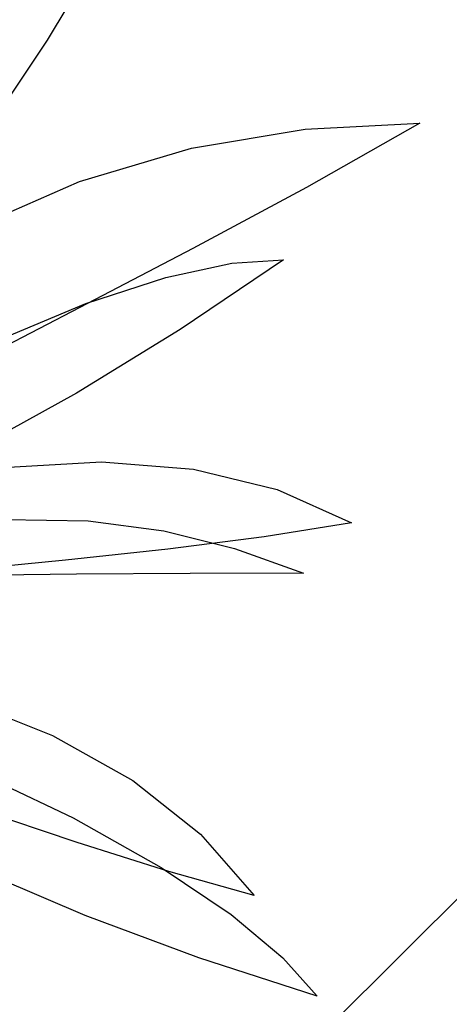
# Model space of a CAD drawing. Units: inches. Extents: x 3590 to 5167, y 65 to 1917.
# Tile 94 of 100: x 5058.39 to 5065.29, y 1773.22 to 1789.03. Entities that reach past the tile are written whole.
import ezdxf

# ---------------------------------------------------------------- set-up
doc = ezdxf.new("R2010")
doc.units = ezdxf.units.IN
for name, color, linetype, lineweight in [('A-ANNO-DIMS', 2, 'Continuous', 18), ('A-FLOR-PATT', 8, 'Continuous', 13), ('L-PLNT', 94, 'Continuous', 18)]:
    doc.layers.add(name, color=color, linetype=linetype, lineweight=lineweight)
doc.layers.add('DIENHOA', color=3, linetype='Continuous')
doc.styles.get("Standard").update_dxf_attribs({"font": 'arial.ttf'})
doc.dimstyles.new('ISO-25', dxfattribs={"dimtxt": 9, "dimasz": 2.5, "dimexe": 1.25, "dimexo": 0.625, "dimtad": 1, "dimdec": 1, "dimlunit": 3, "dimtxsty": 'Standard', "dimcen": 2.5, "dimadec": 0, "dimazin": 0, "dimtfac": 1, "dimtdec": 1, "dimtmove": 0, "dimatfit": 3, "dimfxl": 1, "dimarcsym": 0})

# ---------------------------------------------------------------- blocks, each defined once
blk = doc.blocks.new('Cay03_mb')
at = {"layer": 'DIENHOA'}
for p, q in [((436.81, 297.21), (510.97, 309.61)), ((510.97, 309.61), (585.91, 313.53)), ((585.91, 313.53), (511.78, 271.41)), ((363.38, 275.41), (436.81, 297.21)), ((290.63, 243.24), (363.38, 275.41)), ((511.78, 271.41), (437.63, 231.46)), ((437.63, 231.46), (363.69, 192.89)), ((363.69, 192.89), (290.19, 154.87)), ((314.63, 54.14), (369.18, 53.28)), ((369.18, 53.28), (418.6, 46.82)), ((418.6, 46.82), (464.87, 35.24)), ((464.87, 35.24), (510, 19)), ((361.61, 18.5), (289.03, 17.44)), ((435.8, 18.92), (361.61, 18.5)), ((510, 19), (435.8, 18.92)), ((289.55, -107.64), (359.29, -141.1)), ((359.29, -141.1), (416.89, -173.51)), ((416.89, -173.51), (462.55, -204.2)), ((367.1, -204.83), (296, -174.69)), ((441.55, -232.67), (367.1, -204.83)), ((462.55, -204.2), (496.5, -232.48)), ((518.93, -257.68), (441.55, -232.67)), ((496.5, -232.48), (518.93, -257.68))]:
    blk.add_line(p, q, dxfattribs=at)
for points in [[(384.28, 437.45), (342.25, 367.83), (298.14, 301.71), (252.56, 239.37), (206.11, 181.11), (159.39, 127.21), (113.01, 77.96), (67.57, 33.64), (23.69, -5.44)], [(496.74, 224.01), (429.38, 178.44), (361.6, 136.93), (294.07, 99.46), (227.46, 66.07), (162.44, 36.74), (99.68, 11.49), (39.84, -9.67), (-16.39, -26.73)], [(-16.39, -26.73), (75.38, 37.88), (160.06, 91.82), (237.27, 135.67), (306.57, 170.01), (367.58, 195.44), (419.88, 212.52), (463.07, 221.85), (496.74, 224.01)], [(23.69, -5.44), (99.27, 29.67), (173.22, 57.09), (244.79, 76.69), (313.26, 88.31), (377.88, 91.81), (437.93, 87.02), (492.67, 73.8), (541.37, 52)], [(541.37, 52), (484.11, 42.89), (421.18, 34.83), (354.36, 27.58), (285.41, 20.89), (216.1, 14.49), (148.2, 8.14), (83.47, 1.58), (23.69, -5.44)], [(-16.39, -26.73), (66.95, -26.58), (145.58, -32.71), (218.77, -44.94), (285.79, -63.12), (345.92, -87.06), (398.42, -116.6), (442.57, -151.57), (477.63, -191.79)], [(477.63, -191.79), (421.82, -176.03), (361.32, -156.94), (297.62, -135.49), (232.22, -112.64), (166.63, -89.37), (102.33, -66.65), (40.82, -45.45), (-16.39, -26.73)]]:
    blk.add_lwpolyline(points, dxfattribs=at)
blk = doc.blocks.new('*D322')
at = {"layer": 'A-ANNO-DIMS', "color": 0, "lineweight": -2, "transparency": 16777216}
for p, q in [((5035.744, 1766.184), (5035.744, 1761.199)), ((5064.812, 1766.184), (5064.812, 1761.199)), ((5038.244, 1762.449), (5062.312, 1762.449)), ((5064.812, 1762.449), (5166.991, 1762.449))]:
    blk.add_line(p, q, dxfattribs=at)
at = {"layer": 'A-ANNO-DIMS', "color": 0, "transparency": 16777216}
for points in [[(5038.244, 1762.866), (5038.244, 1762.032), (5035.744, 1762.449)], [(5062.312, 1762.866), (5062.312, 1762.032), (5064.812, 1762.449)]]:
    blk.add_solid(points, dxfattribs=at)
at = {"layer": 'Defpoints', "color": 0, "transparency": 16777216}
for p in [(5035.744, 1766.809), (5064.812, 1766.809), (5064.812, 1762.449)]:
    blk.add_point(p, dxfattribs=at)
at = {"layer": 'A-ANNO-DIMS', "color": 0, "transparency": 16777216, "insert": (5117.152, 1767.669), "char_height": 9, "attachment_point": 5}
blk.add_mtext('PLANT 2\'-5" TYP.', dxfattribs=at)
blk = doc.blocks.new('*D323')
at = {"layer": 'A-ANNO-DIMS', "color": 0, "lineweight": -2, "transparency": 16777216}
for p, q in [((5069.172, 1795.216), (5069.172, 1874.95)), ((5065.437, 1795.216), (5070.422, 1795.216)), ((5069.172, 1769.309), (5069.172, 1792.716)), ((5065.437, 1766.809), (5070.422, 1766.809))]:
    blk.add_line(p, q, dxfattribs=at)
at = {"layer": 'A-ANNO-DIMS', "color": 0, "transparency": 16777216}
for points in [[(5068.756, 1792.716), (5069.589, 1792.716), (5069.172, 1795.216)], [(5068.756, 1769.309), (5069.589, 1769.309), (5069.172, 1766.809)]]:
    blk.add_solid(points, dxfattribs=at)
at = {"layer": 'Defpoints', "color": 0, "transparency": 16777216}
for p in [(5064.812, 1795.216), (5069.172, 1795.216), (5064.812, 1766.809)]:
    blk.add_point(p, dxfattribs=at)
at = {"layer": 'A-ANNO-DIMS', "color": 0, "transparency": 16777216, "insert": (5063.894, 1836.333), "char_height": 9, "attachment_point": 5, "rotation": 90}
blk.add_mtext('2\'-4 1/2" TYP.', dxfattribs=at)

msp = doc.modelspace()

# ---------------------------------------------------------------- hatches: boundary and pattern name
at = {"layer": 'A-FLOR-PATT', "transparency": 33554687}
h = msp.add_hatch(dxfattribs=at)
h.set_pattern_fill('AR-HBONE', color=256, scale=0.2)
h.set_pattern_definition([(45, (-588.972, 0), (0, 28.73682), [60.96, -20.32]), (135, (-574.604, 14.368), (3e-15, 28.73682), [60.96, -20.32])])
h.paths.add_polyline_path([(5071.274, 1796.999), (4933.274, 1796.999), (4933.274, 1753.999), (4962.774, 1753.999, -0.414214), (4928.774, 1719.999), (4933.274, 1718.999), (4933.274, 1334.999), (5071.274, 1334.999)])
h.paths.add_polyline_path([(4951.78, 1521.077), (4951.715, 1521.04), (4951.563, 1520.895)], flags=16)
h.paths.add_polyline_path([(4952.267, 1521.376), (4952.198, 1521.371), (4952.198, 1521.356)], flags=0)
h.paths.add_polyline_path([(4967.051, 1529.728), (4965.231, 1528.694), (4963.411, 1527.714), (4961.756, 1526.851), (4963.589, 1527.449), (4964.036, 1527.478), (4962.975, 1527.249), (4961.76, 1526.852), (4959.792, 1525.834), (4958.005, 1524.895), (4956.24, 1523.93), (4954.504, 1522.919), (4954.129, 1522.682), (4953.361, 1521.997), (4953.366, 1521.998), (4953.605, 1522.064), (4955.106, 1522.761), (4956.921, 1523.434), (4958.678, 1523.915), (4960.358, 1524.2), (4961.945, 1524.286), (4964.171, 1524.108), (4965.958, 1523.309), (4963.863, 1522.976), (4965.187, 1522.499), (4963.366, 1522.497), (4961.545, 1522.487), (4959.764, 1522.461), (4958.304, 1522.419), (4957.974, 1522.388), (4956.307, 1522.232), (4954.718, 1522.071), (4953.251, 1521.899), (4953.525, 1521.623), (4954.331, 1521.379), (4956.243, 1521.23), (4958.039, 1520.93), (4959.684, 1520.483), (4961.16, 1519.896), (4963.107, 1518.8), (4964.393, 1517.325), (4962.973, 1517.726), (4964.558, 1516.661), (4965.407, 1515.708), (4963.507, 1516.322), (4961.68, 1517.005), (4959.935, 1517.745), (4958.282, 1518.528), (4956.732, 1519.343), (4955.295, 1520.175), (4954.672, 1520.572), (4954.513, 1520.627), (4955.658, 1519.318), (4956.703, 1517.982), (4957.644, 1516.647), (4958.485, 1515.334), (4959.55, 1513.524), (4960.438, 1511.769), (4958.841, 1513.62), (4957.452, 1515.325), (4955.819, 1517.459), (4956.665, 1515.448), (4957.111, 1513.923), (4957.447, 1511.714), (4957.076, 1509.793), (4956.538, 1511.11), (4955.992, 1512.569), (4955.444, 1514.125), (4954.898, 1515.735), (4954.357, 1517.356), (4953.824, 1518.943), (4953.305, 1520.452), (4953.065, 1521.116), (4952.971, 1521.146), (4952.949, 1521.086), (4952.73, 1520.199), (4953.37, 1518.024), (4953.757, 1516.373), (4954.051, 1514.765), (4954.264, 1513.221), (4954.471, 1511.131), (4954.497, 1510.402), (4954.409, 1511.76), (4954.264, 1513.221), (4954.051, 1514.765), (4953.757, 1516.373), (4953.37, 1518.024), (4952.877, 1519.698), (4952.716, 1520.141), (4952.533, 1519.059), (4952.374, 1517.789), (4952.219, 1516.312), (4952.046, 1514.6), (4951.833, 1512.626), (4951.557, 1510.363), (4951.203, 1512.168), (4950.852, 1514.339), (4950.985, 1516.376), (4951.66, 1518.286), (4952.593, 1520.481), (4952.357, 1521.13), (4951.855, 1520.328), (4950.839, 1518.908), (4949.777, 1517.587), (4948.916, 1516.617), (4948.111, 1515.256), (4947.089, 1513.554), (4945.889, 1511.615), (4946.326, 1513.402), (4946.562, 1514.249), (4945.528, 1513.327), (4944.581, 1512.531), (4946.018, 1514.508), (4947.204, 1516.048), (4947.893, 1517.313), (4949.307, 1518.764), (4950.414, 1519.767), (4950.451, 1519.806), (4952.267, 1521.376), (4951.645, 1521.493), (4950.404, 1521.18), (4948.044, 1520.359), (4946.119, 1519.452), (4944.572, 1518.475), (4943.35, 1517.443), (4941.997, 1515.92), (4941.661, 1515.275), (4942.813, 1516.99), (4944.572, 1518.475), (4946.119, 1519.452), (4948.044, 1520.359), (4950.404, 1521.18), (4951.645, 1521.493), (4949.647, 1521.868), (4948.6, 1521.756), (4947.126, 1521.57), (4945.42, 1521.348), (4943.45, 1521.105), (4941.183, 1520.856), (4942.86, 1521.613), (4943.873, 1522.03), (4942.952, 1521.909), (4941.41, 1521.485), (4939.543, 1520.67), (4938.968, 1520.226), (4940.733, 1521.299), (4942.952, 1521.909), (4943.702, 1522.008), (4945.894, 1522.7), (4947.565, 1522.714), (4948.921, 1522.566), (4951.131, 1522.183), (4950.971, 1522.297), (4948.129, 1523.006), (4946.035, 1523.707), (4944.232, 1524.521), (4942.707, 1525.461), (4941.444, 1526.537), (4940.43, 1527.761), (4939.649, 1529.143), (4941.421, 1528.122), (4943.147, 1527.132), (4944.841, 1526.175), (4946.514, 1525.25), (4948.179, 1524.359), (4948.365, 1524.263), (4946.475, 1526.045), (4945.181, 1527.54), (4944.19, 1529.033), (4943.496, 1530.54), (4943.278, 1531.36), (4942.498, 1531.919), (4943.114, 1531.762), (4942.959, 1533.659), (4944.14, 1531.989), (4944.612, 1531.323), (4946.202, 1530.463), (4947.486, 1529.509), (4948.79, 1528.226), (4950.368, 1526.237), (4949.485, 1528.155), (4948.851, 1530.123), (4948.491, 1532.041), (4948.381, 1533.918), (4948.501, 1535.76), (4948.827, 1537.573), (4949.418, 1535.565), (4949.957, 1533.569), (4950.464, 1531.586), (4950.961, 1529.617), (4951.391, 1527.954), (4951.724, 1530.687), (4952.201, 1532.58), (4952.889, 1534.33), (4953.77, 1535.951), (4954.827, 1537.46), (4954.521, 1535.39), (4954.273, 1533.937), (4955.58, 1535.663), (4956.748, 1536.739), (4956.159, 1534.78), (4955.589, 1532.873), (4955.043, 1531.006), (4954.525, 1529.166), (4954.038, 1527.341), (4953.638, 1525.733), (4953.611, 1525.586), (4953.398, 1524.166), (4953.382, 1524.009), (4954.07, 1525.476), (4954.912, 1527.022), (4956.136, 1528.894), (4957.847, 1530.577), (4959.376, 1531.54), (4958.256, 1530.104), (4957.143, 1528.663), (4956.066, 1527.243), (4955.056, 1525.871), (4954.141, 1524.571), (4953.352, 1523.372), (4953.311, 1523.303), (4953.273, 1522.925), (4953.261, 1522.382), (4954.103, 1523.373), (4954.63, 1524.284), (4955.961, 1526.358), (4957.23, 1528.13), (4958.421, 1529.609), (4960.037, 1531.368), (4961.374, 1532.375), (4962.101, 1532.77), (4961.07, 1531.061), (4959.987, 1529.438), (4958.869, 1527.908), (4958.15, 1527.007), (4959.803, 1528.003), (4961.589, 1528.793), (4963.391, 1529.328), (4965.211, 1529.632)], flags=16)
h.paths.add_polyline_path([(4962.944, 1523.182), (4961.107, 1523.422), (4960.392, 1523.362), (4962.35, 1523.331)], flags=0)
h.paths.add_polyline_path([(5049.541, 1584.551), (5049.476, 1584.515), (5049.325, 1584.37)], flags=16)
h.paths.add_polyline_path([(5050.028, 1584.851), (5049.959, 1584.845), (5049.959, 1584.83)], flags=0)
h.paths.add_polyline_path([(5042.333, 1581.949), (5043.88, 1582.926), (5045.806, 1583.833), (5048.165, 1584.654), (5049.406, 1584.967), (5047.408, 1585.342), (5046.361, 1585.231), (5044.888, 1585.044), (5043.181, 1584.822), (5041.211, 1584.579), (5038.944, 1584.33), (5040.622, 1585.087), (5041.634, 1585.504), (5040.713, 1585.383), (5039.171, 1584.959), (5037.304, 1584.144), (5036.729, 1583.7), (5038.494, 1584.773), (5040.713, 1585.383), (5041.463, 1585.482), (5043.655, 1586.174), (5045.326, 1586.188), (5046.682, 1586.04), (5048.893, 1585.657), (5048.732, 1585.771), (5045.891, 1586.48), (5043.796, 1587.181), (5041.994, 1587.996), (5040.468, 1588.935), (5039.205, 1590.011), (5038.191, 1591.235), (5037.41, 1592.617), (5039.182, 1591.596), (5040.909, 1590.607), (5042.602, 1589.649), (5044.275, 1588.724), (5045.94, 1587.833), (5046.126, 1587.738), (5044.237, 1589.519), (5042.942, 1591.015), (5041.952, 1592.508), (5041.257, 1594.014), (5041.039, 1594.834), (5040.26, 1595.393), (5040.875, 1595.237), (5040.721, 1597.133), (5041.901, 1595.463), (5042.373, 1594.798), (5043.963, 1593.938), (5045.247, 1592.983), (5046.552, 1591.701), (5048.129, 1589.712), (5047.247, 1591.63), (5046.613, 1593.597), (5046.252, 1595.515), (5046.142, 1597.392), (5046.262, 1599.234), (5046.588, 1601.047), (5047.179, 1599.039), (5047.718, 1597.043), (5048.225, 1595.06), (5048.722, 1593.091), (5049.152, 1591.429), (5049.485, 1594.161), (5049.962, 1596.054), (5050.65, 1597.804), (5051.532, 1599.425), (5052.589, 1600.934), (5052.283, 1598.864), (5052.034, 1597.411), (5053.341, 1599.137), (5054.509, 1600.213), (5053.92, 1598.254), (5053.35, 1596.348), (5052.805, 1594.48), (5052.286, 1592.64), (5051.799, 1590.815), (5051.4, 1589.207), (5051.373, 1589.06), (5051.159, 1587.64), (5051.143, 1587.483), (5051.831, 1588.95), (5052.673, 1590.496), (5053.898, 1592.368), (5055.608, 1594.051), (5057.137, 1595.014), (5056.017, 1593.578), (5054.904, 1592.137), (5053.828, 1590.717), (5052.817, 1589.345), (5051.902, 1588.046), (5051.113, 1586.846), (5051.072, 1586.777), (5051.034, 1586.399), (5051.022, 1585.856), (5051.864, 1586.847), (5052.391, 1587.758), (5053.723, 1589.832), (5054.991, 1591.604), (5056.182, 1593.083), (5057.798, 1594.842), (5059.135, 1595.849), (5059.863, 1596.244), (5058.831, 1594.535), (5057.749, 1592.912), (5056.63, 1591.382), (5055.912, 1590.482), (5057.564, 1591.477), (5059.35, 1592.267), (5061.152, 1592.802), (5062.972, 1593.106), (5064.812, 1593.203), (5062.992, 1592.169), (5061.172, 1591.188), (5059.518, 1590.325), (5061.35, 1590.924), (5061.797, 1590.952), (5060.737, 1590.723), (5059.521, 1590.326), (5057.553, 1589.308), (5055.766, 1588.369), (5054.002, 1587.404), (5052.265, 1586.393), (5051.891, 1586.156), (5051.122, 1585.471), (5051.127, 1585.472), (5051.366, 1585.538), (5052.867, 1586.235), (5054.682, 1586.908), (5056.439, 1587.389), (5058.12, 1587.675), (5059.706, 1587.76), (5061.933, 1587.583), (5063.719, 1586.783), (5061.624, 1586.45), (5062.949, 1585.973), (5061.127, 1585.971), (5059.307, 1585.961), (5057.525, 1585.935), (5056.065, 1585.893), (5055.735, 1585.862), (5054.068, 1585.707), (5052.479, 1585.546), (5051.012, 1585.373), (5051.286, 1585.097), (5052.092, 1584.853), (5054.004, 1584.704), (5055.8, 1584.404), (5057.446, 1583.958), (5058.921, 1583.37), (5060.868, 1582.274), (5062.154, 1580.799), (5060.734, 1581.2), (5062.32, 1580.135), (5063.168, 1579.182), (5061.269, 1579.796), (5059.441, 1580.479), (5057.696, 1581.219), (5056.043, 1582.003), (5054.493, 1582.817), (5053.057, 1583.649), (5052.433, 1584.047), (5052.274, 1584.101), (5053.42, 1582.793), (5054.464, 1581.457), (5055.405, 1580.121), (5056.247, 1578.809), (5057.311, 1576.998), (5058.199, 1575.244), (5056.602, 1577.094), (5055.213, 1578.799), (5053.58, 1580.933), (5054.427, 1578.922), (5054.872, 1577.397), (5055.208, 1575.189), (5054.838, 1573.267), (5054.299, 1574.584), (5053.754, 1576.043), (5053.206, 1577.599), (5052.659, 1579.209), (5052.118, 1580.83), (5051.585, 1582.417), (5051.066, 1583.927), (5050.826, 1584.59), (5050.733, 1584.62), (5050.711, 1584.561), (5050.491, 1583.673), (5051.131, 1581.498), (5051.518, 1579.847), (5051.813, 1578.24), (5052.026, 1576.695), (5052.233, 1574.605), (5052.258, 1573.876), (5052.17, 1575.234), (5052.026, 1576.695), (5051.813, 1578.24), (5051.518, 1579.847), (5051.131, 1581.498), (5050.638, 1583.172), (5050.477, 1583.615), (5050.294, 1582.533), (5050.136, 1581.263), (5049.981, 1579.786), (5049.807, 1578.074), (5049.594, 1576.1), (5049.318, 1573.837), (5048.965, 1575.642), (5048.613, 1577.813), (5048.747, 1579.85), (5049.421, 1581.76), (5050.354, 1583.955), (5050.118, 1584.604), (5049.616, 1583.802), (5048.6, 1582.382), (5047.538, 1581.061), (5046.677, 1580.091), (5045.872, 1578.73), (5044.85, 1577.028), (5043.651, 1575.089), (5044.087, 1576.877), (5044.324, 1577.723), (5043.289, 1576.801), (5042.342, 1576.005), (5043.779, 1577.982), (5044.966, 1579.522), (5045.655, 1580.787), (5047.068, 1582.239), (5048.175, 1583.241), (5048.213, 1583.28), (5050.028, 1584.851), (5049.406, 1584.967), (5048.165, 1584.654), (5045.806, 1583.833), (5043.88, 1582.926), (5042.333, 1581.949), (5041.111, 1580.917), (5039.758, 1579.394), (5039.423, 1578.749), (5040.575, 1580.464)], flags=16)
h.paths.add_polyline_path([(4954.799, 1533.12), (4954.262, 1532.079), (4953.831, 1530.935), (4953.505, 1529.636), (4953.283, 1528.133), (4953.167, 1526.376), (4953.156, 1524.315), (4953.277, 1521.236), (4952.802, 1521.842), (4951.557, 1521.998), (4950.976, 1521.961), (4952.661, 1521.941), (4952.802, 1521.842), (4953.152, 1523.593), (4953.167, 1526.376), (4953.283, 1528.133), (4953.609, 1530.346), (4954.456, 1532.592)], flags=0)
h.paths.add_polyline_path([(5050.563, 1585.316), (5049.318, 1585.472), (5048.737, 1585.435), (5050.422, 1585.415), (5050.563, 1585.316), (5050.914, 1587.067), (5050.928, 1589.851), (5051.045, 1591.607), (5051.371, 1593.82), (5052.217, 1596.066), (5052.56, 1596.594), (5052.024, 1595.554), (5051.592, 1594.409), (5051.266, 1593.11), (5051.045, 1591.607), (5050.928, 1589.851), (5050.918, 1587.789), (5051.038, 1584.71)], flags=0)
h.paths.add_polyline_path([(5058.153, 1586.836), (5060.111, 1586.805), (5060.705, 1586.656), (5058.868, 1586.896)], flags=0)
h.paths.add_polyline_path([(5049.541, 1430.936), (5049.476, 1430.9), (5049.325, 1430.755)], flags=16)
h.paths.add_polyline_path([(5050.028, 1431.236), (5049.959, 1431.231), (5049.959, 1431.215)], flags=0)
h.paths.add_polyline_path([(5046.588, 1447.432), (5047.179, 1445.425), (5047.718, 1443.429), (5048.225, 1441.446), (5048.722, 1439.476), (5049.152, 1437.814), (5049.485, 1440.546), (5049.962, 1442.439), (5050.65, 1444.189), (5051.532, 1445.811), (5052.589, 1447.319), (5052.283, 1445.249), (5052.034, 1443.796), (5053.341, 1445.522), (5054.509, 1446.598), (5053.92, 1444.64), (5053.35, 1442.733), (5052.805, 1440.865), (5052.286, 1439.025), (5051.799, 1437.201), (5051.4, 1435.592), (5051.373, 1435.445), (5051.159, 1434.025), (5051.143, 1433.868), (5051.831, 1435.335), (5052.673, 1436.881), (5053.898, 1438.753), (5055.608, 1440.436), (5057.137, 1441.4), (5056.017, 1439.963), (5054.904, 1438.522), (5053.828, 1437.102), (5052.817, 1435.73), (5051.902, 1434.431), (5051.113, 1433.231), (5051.072, 1433.162), (5051.034, 1432.784), (5051.022, 1432.242), (5051.864, 1433.232), (5052.391, 1434.143), (5053.723, 1436.217), (5054.991, 1437.989), (5056.182, 1439.468), (5057.798, 1441.227), (5059.135, 1442.235), (5059.863, 1442.629), (5058.831, 1440.921), (5057.749, 1439.298), (5056.63, 1437.767), (5055.912, 1436.867), (5057.564, 1437.863), (5059.35, 1438.652), (5061.152, 1439.187), (5062.972, 1439.491), (5064.812, 1439.588), (5062.992, 1438.554), (5061.172, 1437.573), (5059.518, 1436.71), (5061.35, 1437.309), (5061.797, 1437.337), (5060.737, 1437.108), (5059.521, 1436.711), (5057.553, 1435.693), (5055.766, 1434.754), (5054.002, 1433.789), (5052.265, 1432.778), (5051.891, 1432.541), (5051.122, 1431.856), (5051.127, 1431.857), (5051.366, 1431.923), (5052.867, 1432.62), (5054.682, 1433.293), (5056.439, 1433.775), (5058.12, 1434.06), (5059.706, 1434.145), (5061.933, 1433.968), (5063.719, 1433.168), (5061.624, 1432.835), (5062.949, 1432.358), (5061.127, 1432.357), (5059.307, 1432.346), (5057.525, 1432.32), (5056.065, 1432.278), (5055.735, 1432.248), (5054.068, 1432.092), (5052.479, 1431.931), (5051.012, 1431.759), (5051.286, 1431.482), (5052.092, 1431.238), (5054.004, 1431.089), (5055.8, 1430.789), (5057.446, 1430.343), (5058.921, 1429.755), (5060.868, 1428.66), (5062.154, 1427.185), (5060.734, 1427.585), (5062.32, 1426.52), (5063.168, 1425.567), (5061.269, 1426.181), (5059.441, 1426.865), (5057.696, 1427.604), (5056.043, 1428.388), (5054.493, 1429.202), (5053.057, 1430.034), (5052.433, 1430.432), (5052.274, 1430.487), (5053.42, 1429.178), (5054.464, 1427.842), (5055.405, 1426.506), (5056.247, 1425.194), (5057.311, 1423.383), (5058.199, 1421.629), (5056.602, 1423.479), (5055.213, 1425.184), (5053.58, 1427.318), (5054.427, 1425.307), (5054.872, 1423.782), (5055.208, 1421.574), (5054.838, 1419.652), (5054.299, 1420.97), (5053.754, 1422.428), (5053.206, 1423.984), (5052.659, 1425.595), (5052.118, 1427.215), (5051.585, 1428.802), (5051.066, 1430.312), (5050.826, 1430.975), (5050.733, 1431.005), (5050.711, 1430.946), (5050.491, 1430.058), (5051.131, 1427.883), (5051.518, 1426.232), (5051.813, 1424.625), (5052.026, 1423.081), (5052.233, 1420.991), (5052.258, 1420.261), (5052.17, 1421.619), (5052.026, 1423.081), (5051.813, 1424.625), (5051.518, 1426.232), (5051.131, 1427.883), (5050.638, 1429.558), (5050.477, 1430.001), (5050.294, 1428.918), (5050.136, 1427.648), (5049.981, 1426.171), (5049.807, 1424.459), (5049.594, 1422.485), (5049.318, 1420.222), (5048.965, 1422.028), (5048.613, 1424.199), (5048.747, 1426.235), (5049.421, 1428.146), (5050.354, 1430.34), (5050.118, 1430.989), (5049.616, 1430.187), (5048.6, 1428.768), (5047.538, 1427.446), (5046.677, 1426.477), (5045.872, 1425.116), (5044.85, 1423.413), (5043.651, 1421.474), (5044.087, 1423.262), (5044.324, 1424.109), (5043.289, 1423.186), (5042.342, 1422.391), (5043.779, 1424.368), (5044.966, 1425.907), (5045.655, 1427.173), (5047.068, 1428.624), (5048.175, 1429.627), (5048.213, 1429.666), (5050.028, 1431.236), (5049.406, 1431.353), (5048.165, 1431.039), (5045.806, 1430.218), (5043.88, 1429.311), (5042.333, 1428.334), (5041.111, 1427.302), (5039.758, 1425.779), (5039.423, 1425.134), (5040.575, 1426.849), (5042.333, 1428.334), (5043.88, 1429.311), (5045.806, 1430.218), (5048.165, 1431.039), (5049.406, 1431.353), (5047.408, 1431.727), (5046.361, 1431.616), (5044.888, 1431.429), (5043.181, 1431.207), (5041.211, 1430.964), (5038.944, 1430.715), (5040.622, 1431.472), (5041.634, 1431.89), (5040.713, 1431.769), (5039.171, 1431.345), (5037.304, 1430.53), (5036.729, 1430.085), (5038.494, 1431.158), (5040.713, 1431.769), (5041.463, 1431.867), (5043.655, 1432.559), (5045.326, 1432.573), (5046.682, 1432.425), (5048.893, 1432.042), (5048.732, 1432.156), (5045.891, 1432.865), (5043.796, 1433.566), (5041.994, 1434.381), (5040.468, 1435.321), (5039.205, 1436.396), (5038.191, 1437.62), (5037.41, 1439.002), (5039.182, 1437.982), (5040.909, 1436.992), (5042.602, 1436.034), (5044.275, 1435.109), (5045.94, 1434.218), (5046.126, 1434.123), (5044.237, 1435.904), (5042.942, 1437.4), (5041.952, 1438.893), (5041.257, 1440.399), (5041.039, 1441.219), (5040.26, 1441.778), (5040.875, 1441.622), (5040.721, 1443.518), (5041.901, 1441.848), (5042.373, 1441.183), (5043.963, 1440.323), (5045.247, 1439.369), (5046.552, 1438.086), (5048.129, 1436.097), (5047.247, 1438.015), (5046.613, 1439.982), (5046.252, 1441.901), (5046.142, 1443.778), (5046.262, 1445.619)], flags=16)
h.paths.add_polyline_path([(5052.382, 1444.255), (5051.623, 1442.78), (5052.024, 1441.939), (5052.56, 1442.98)], flags=0)
h.paths.add_polyline_path([(5050.563, 1431.701), (5049.318, 1431.857), (5048.737, 1431.821), (5050.422, 1431.8)], flags=0)
h.paths.add_polyline_path([(5058.153, 1433.221), (5060.111, 1433.19), (5060.705, 1433.041), (5058.868, 1433.281)], flags=0)
h.paths.add_polyline_path([(5049.541, 1352.285), (5049.476, 1352.249), (5049.325, 1352.104)], flags=16)
h.paths.add_polyline_path([(5050.028, 1352.585), (5049.959, 1352.58), (5049.959, 1352.564)], flags=0)
h.paths.add_polyline_path([(5046.588, 1368.781), (5047.179, 1366.774), (5047.718, 1364.778), (5048.225, 1362.795), (5048.722, 1360.825), (5049.152, 1359.163), (5049.485, 1361.896), (5049.962, 1363.789), (5050.65, 1365.538), (5051.532, 1367.16), (5052.589, 1368.669), (5052.283, 1366.598), (5052.034, 1365.145), (5053.341, 1366.871), (5054.509, 1367.947), (5053.92, 1365.989), (5053.35, 1364.082), (5052.805, 1362.214), (5052.286, 1360.374), (5051.799, 1358.55), (5051.4, 1356.942), (5051.373, 1356.794), (5051.159, 1355.374), (5051.143, 1355.218), (5051.831, 1356.684), (5052.673, 1358.23), (5053.898, 1360.102), (5055.608, 1361.786), (5057.137, 1362.749), (5056.017, 1361.313), (5054.904, 1359.872), (5053.828, 1358.452), (5052.817, 1357.079), (5051.902, 1355.78), (5051.113, 1354.581), (5051.072, 1354.512), (5051.034, 1354.133), (5051.022, 1353.591), (5051.864, 1354.581), (5052.391, 1355.492), (5053.723, 1357.566), (5054.991, 1359.338), (5056.182, 1360.817), (5057.798, 1362.577), (5059.135, 1363.584), (5059.863, 1363.979), (5058.831, 1362.27), (5057.749, 1360.647), (5056.63, 1359.117), (5055.912, 1358.216), (5057.564, 1359.212), (5059.35, 1360.001), (5061.152, 1360.536), (5062.972, 1360.841), (5064.812, 1360.937), (5062.992, 1359.903), (5061.172, 1358.923), (5059.518, 1358.059), (5061.35, 1358.658), (5061.797, 1358.687), (5060.737, 1358.458), (5059.521, 1358.061), (5057.553, 1357.043), (5055.766, 1356.103), (5054.002, 1355.138), (5052.265, 1354.127), (5051.891, 1353.89), (5051.122, 1353.206), (5051.127, 1353.206), (5051.366, 1353.272), (5052.867, 1353.969), (5054.682, 1354.643), (5056.439, 1355.124), (5058.12, 1355.409), (5059.706, 1355.495), (5061.933, 1355.317), (5063.719, 1354.518), (5061.624, 1354.184), (5062.949, 1353.708), (5061.127, 1353.706), (5059.307, 1353.695), (5057.525, 1353.669), (5056.065, 1353.627), (5055.735, 1353.597), (5054.068, 1353.441), (5052.479, 1353.28), (5051.012, 1353.108), (5051.286, 1352.831), (5052.092, 1352.587), (5054.004, 1352.439), (5055.8, 1352.138), (5057.446, 1351.692), (5058.921, 1351.104), (5060.868, 1350.009), (5062.154, 1348.534), (5060.734, 1348.935), (5062.32, 1347.869), (5063.168, 1346.916), (5061.269, 1347.53), (5059.441, 1348.214), (5057.696, 1348.954), (5056.043, 1349.737), (5054.493, 1350.551), (5053.057, 1351.383), (5052.433, 1351.781), (5052.274, 1351.836), (5053.42, 1350.527), (5054.464, 1349.191), (5055.405, 1347.855), (5056.247, 1346.543), (5057.311, 1344.733), (5058.199, 1342.978), (5056.602, 1344.828), (5055.213, 1346.534), (5053.58, 1348.667), (5054.427, 1346.656), (5054.872, 1345.132), (5055.208, 1342.923), (5054.838, 1341.002), (5054.299, 1342.319), (5053.754, 1343.778), (5053.206, 1345.334), (5052.659, 1346.944), (5052.118, 1348.564), (5051.585, 1350.151), (5051.066, 1351.661), (5050.826, 1352.324), (5050.733, 1352.355), (5050.711, 1352.295), (5050.491, 1351.408), (5051.131, 1349.232), (5051.518, 1347.581), (5051.813, 1345.974), (5052.026, 1344.43), (5052.233, 1342.34), (5052.258, 1341.61), (5052.17, 1342.969), (5052.026, 1344.43), (5051.813, 1345.974), (5051.518, 1347.581), (5051.131, 1349.232), (5050.638, 1350.907), (5050.477, 1351.35), (5050.294, 1350.267), (5050.136, 1348.997), (5049.981, 1347.52), (5049.807, 1345.809), (5049.594, 1343.835), (5049.318, 1341.571), (5048.965, 1343.377), (5048.613, 1345.548), (5048.747, 1347.585), (5049.421, 1349.495), (5050.354, 1351.689), (5050.118, 1352.339), (5049.616, 1351.536), (5048.6, 1350.117), (5047.538, 1348.795), (5046.677, 1347.826), (5045.872, 1346.465), (5044.85, 1344.763), (5043.651, 1342.824), (5044.087, 1344.611), (5044.324, 1345.458), (5043.289, 1344.535), (5042.342, 1343.74), (5043.779, 1345.717), (5044.966, 1347.256), (5045.655, 1348.522), (5047.068, 1349.973), (5048.175, 1350.976), (5048.213, 1351.015), (5050.028, 1352.585), (5049.406, 1352.702), (5048.165, 1352.388), (5045.806, 1351.567), (5043.88, 1350.661), (5042.333, 1349.683), (5041.111, 1348.651), (5039.758, 1347.128), (5039.423, 1346.483), (5040.575, 1348.198), (5042.333, 1349.683), (5043.88, 1350.661), (5045.806, 1351.567), (5048.165, 1352.388), (5049.406, 1352.702), (5047.408, 1353.076), (5046.361, 1352.965), (5044.888, 1352.779), (5043.181, 1352.556), (5041.211, 1352.313), (5038.944, 1352.065), (5040.622, 1352.821), (5041.634, 1353.239), (5040.713, 1353.118), (5039.171, 1352.694), (5037.304, 1351.879), (5036.729, 1351.434), (5038.494, 1352.508), (5040.713, 1353.118), (5041.463, 1353.216), (5043.655, 1353.909), (5045.326, 1353.923), (5046.682, 1353.774), (5048.893, 1353.391), (5048.732, 1353.506), (5045.891, 1354.214), (5043.796, 1354.915), (5041.994, 1355.73), (5040.468, 1356.67), (5039.205, 1357.746), (5038.191, 1358.969), (5037.41, 1360.352), (5039.182, 1359.331), (5040.909, 1358.341), (5042.602, 1357.383), (5044.275, 1356.458), (5045.94, 1355.567), (5046.126, 1355.472), (5044.237, 1357.253), (5042.942, 1358.749), (5041.952, 1360.242), (5041.257, 1361.748), (5041.039, 1362.568), (5040.26, 1363.128), (5040.875, 1362.971), (5040.721, 1364.867), (5041.901, 1363.197), (5042.373, 1362.532), (5043.963, 1361.672), (5045.247, 1360.718), (5046.552, 1359.435), (5048.129, 1357.446), (5047.247, 1359.364), (5046.613, 1361.331), (5046.252, 1363.25), (5046.142, 1365.127), (5046.262, 1366.969)], flags=16)
h.paths.add_polyline_path([(5052.382, 1365.604), (5051.623, 1364.129), (5052.024, 1363.288), (5052.56, 1364.329)], flags=0)
h.paths.add_polyline_path([(4951.78, 1698.041), (4951.715, 1698.005), (4951.563, 1697.859)], flags=16)
h.paths.add_polyline_path([(4952.267, 1698.341), (4952.198, 1698.335), (4952.198, 1698.32)], flags=0)
h.paths.add_polyline_path([(4957.076, 1686.757), (4956.538, 1688.074), (4955.992, 1689.533), (4955.444, 1691.089), (4954.898, 1692.699), (4954.357, 1694.32), (4953.824, 1695.907), (4953.305, 1697.417), (4953.065, 1698.08), (4952.971, 1698.11), (4952.949, 1698.051), (4952.73, 1697.163), (4953.37, 1694.988), (4953.757, 1693.337), (4954.051, 1691.729), (4954.264, 1690.185), (4954.471, 1688.095), (4954.497, 1687.366), (4954.409, 1688.724), (4954.264, 1690.185), (4954.051, 1691.729), (4953.757, 1693.337), (4953.37, 1694.988), (4952.877, 1696.662), (4952.716, 1697.105), (4952.533, 1696.023), (4952.374, 1694.753), (4952.219, 1693.276), (4952.046, 1691.564), (4951.833, 1689.59), (4951.557, 1687.327), (4951.203, 1689.132), (4950.852, 1691.303), (4950.985, 1693.34), (4951.66, 1695.25), (4952.593, 1697.445), (4952.357, 1698.094), (4951.855, 1697.292), (4950.839, 1695.872), (4949.777, 1694.551), (4948.916, 1693.581), (4948.111, 1692.22), (4947.089, 1690.518), (4945.889, 1688.579), (4946.326, 1690.366), (4946.562, 1691.213), (4945.528, 1690.291), (4944.581, 1689.495), (4946.018, 1691.472), (4947.204, 1693.012), (4947.893, 1694.277), (4949.307, 1695.729), (4950.414, 1696.731), (4950.451, 1696.77), (4952.267, 1698.341), (4951.645, 1698.457), (4950.404, 1698.144), (4948.044, 1697.323), (4946.119, 1696.416), (4944.572, 1695.439), (4943.35, 1694.407), (4941.997, 1692.884), (4941.661, 1692.239), (4942.813, 1693.954), (4944.572, 1695.439), (4946.119, 1696.416), (4948.044, 1697.323), (4950.404, 1698.144), (4951.645, 1698.457), (4949.647, 1698.832), (4948.6, 1698.72), (4947.126, 1698.534), (4945.42, 1698.312), (4943.45, 1698.069), (4941.183, 1697.82), (4942.86, 1698.577), (4943.873, 1698.994), (4942.952, 1698.873), (4941.41, 1698.449), (4939.543, 1697.634), (4938.968, 1697.19), (4940.733, 1698.263), (4942.952, 1698.873), (4943.702, 1698.972), (4945.894, 1699.664), (4947.565, 1699.678), (4948.921, 1699.53), (4951.131, 1699.147), (4950.971, 1699.261), (4948.129, 1699.97), (4946.035, 1700.671), (4944.232, 1701.486), (4942.707, 1702.425), (4941.444, 1703.501), (4940.43, 1704.725), (4939.649, 1706.107), (4941.421, 1705.086), (4943.147, 1704.097), (4944.841, 1703.139), (4946.514, 1702.214), (4948.179, 1701.323), (4948.365, 1701.227), (4946.475, 1703.009), (4945.181, 1704.505), (4944.19, 1705.997), (4943.496, 1707.504), (4943.278, 1708.324), (4942.498, 1708.883), (4943.114, 1708.727), (4942.959, 1710.623), (4944.14, 1708.953), (4944.612, 1708.287), (4946.202, 1707.428), (4947.486, 1706.473), (4948.79, 1705.191), (4950.368, 1703.202), (4949.485, 1705.12), (4948.851, 1707.087), (4948.491, 1709.005), (4948.381, 1710.882), (4948.501, 1712.724), (4948.827, 1714.537), (4949.418, 1712.529), (4949.957, 1710.533), (4950.464, 1708.55), (4950.961, 1706.581), (4951.391, 1704.919), (4951.724, 1707.651), (4952.201, 1709.544), (4952.889, 1711.294), (4953.77, 1712.915), (4954.827, 1714.424), (4954.521, 1712.354), (4954.273, 1710.901), (4955.58, 1712.627), (4956.748, 1713.703), (4956.159, 1711.744), (4955.589, 1709.837), (4955.043, 1707.97), (4954.525, 1706.13), (4954.038, 1704.305), (4953.638, 1702.697), (4953.611, 1702.55), (4953.398, 1701.13), (4953.382, 1700.973), (4954.07, 1702.44), (4954.912, 1703.986), (4956.136, 1705.858), (4957.847, 1707.541), (4959.376, 1708.504), (4958.256, 1707.068), (4957.143, 1705.627), (4956.066, 1704.207), (4955.056, 1702.835), (4954.141, 1701.536), (4953.352, 1700.336), (4953.311, 1700.267), (4953.273, 1699.889), (4953.261, 1699.346), (4954.103, 1700.337), (4954.63, 1701.248), (4955.961, 1703.322), (4957.23, 1705.094), (4958.421, 1706.573), (4960.037, 1708.332), (4961.374, 1709.339), (4962.101, 1709.734), (4961.07, 1708.025), (4959.987, 1706.402), (4958.869, 1704.872), (4958.15, 1703.972), (4959.803, 1704.967), (4961.589, 1705.757), (4963.391, 1706.292), (4965.211, 1706.596), (4967.051, 1706.692), (4965.231, 1705.659), (4963.411, 1704.678), (4961.756, 1703.815), (4963.589, 1704.413), (4964.036, 1704.442), (4962.975, 1704.213), (4961.76, 1703.816), (4959.792, 1702.798), (4958.005, 1701.859), (4956.24, 1700.894), (4954.504, 1699.883), (4954.129, 1699.646), (4953.361, 1698.961), (4953.366, 1698.962), (4953.605, 1699.028), (4955.106, 1699.725), (4956.921, 1700.398), (4958.678, 1700.879), (4960.358, 1701.164), (4961.945, 1701.25), (4964.171, 1701.073), (4965.958, 1700.273), (4963.863, 1699.94), (4965.187, 1699.463), (4963.366, 1699.461), (4961.545, 1699.451), (4959.764, 1699.425), (4958.304, 1699.383), (4957.974, 1699.352), (4956.307, 1699.197), (4954.718, 1699.036), (4953.251, 1698.863), (4953.525, 1698.587), (4954.331, 1698.343), (4956.243, 1698.194), (4958.039, 1697.894), (4959.684, 1697.447), (4961.16, 1696.86), (4963.107, 1695.764), (4964.393, 1694.289), (4962.973, 1694.69), (4964.558, 1693.625), (4965.407, 1692.672), (4963.507, 1693.286), (4961.68, 1693.969), (4959.935, 1694.709), (4958.282, 1695.492), (4956.732, 1696.307), (4955.295, 1697.139), (4954.672, 1697.536), (4954.513, 1697.591), (4955.658, 1696.282), (4956.703, 1694.946), (4957.644, 1693.611), (4958.485, 1692.298), (4959.55, 1690.488), (4960.438, 1688.733), (4958.841, 1690.584), (4957.452, 1692.289), (4955.819, 1694.423), (4956.665, 1692.412), (4957.111, 1690.887), (4957.447, 1688.678)], flags=16)
h.paths.add_polyline_path([(5050.563, 1353.05), (5049.318, 1353.207), (5048.737, 1353.17), (5050.422, 1353.15)], flags=0)
h.paths.add_polyline_path([(4951.78, 1351.486), (4951.715, 1351.45), (4951.563, 1351.305)], flags=16)
h.paths.add_polyline_path([(4952.267, 1351.786), (4952.198, 1351.78), (4952.198, 1351.765)], flags=0)
h.paths.add_polyline_path([(4954.827, 1367.869), (4954.521, 1365.799), (4954.273, 1364.346), (4955.58, 1366.072), (4956.748, 1367.148), (4956.159, 1365.19), (4955.589, 1363.283), (4955.043, 1361.415), (4954.525, 1359.575), (4954.038, 1357.751), (4953.638, 1356.142), (4953.611, 1355.995), (4953.398, 1354.575), (4953.382, 1354.418), (4954.07, 1355.885), (4954.912, 1357.431), (4956.136, 1359.303), (4957.847, 1360.986), (4959.376, 1361.95), (4958.256, 1360.513), (4957.143, 1359.072), (4956.066, 1357.652), (4955.056, 1356.28), (4954.141, 1354.981), (4953.352, 1353.781), (4953.311, 1353.712), (4953.273, 1353.334), (4953.261, 1352.792), (4954.103, 1353.782), (4954.63, 1354.693), (4955.961, 1356.767), (4957.23, 1358.539), (4958.421, 1360.018), (4960.037, 1361.777), (4961.374, 1362.785), (4962.101, 1363.179), (4961.07, 1361.471), (4959.987, 1359.848), (4958.869, 1358.317), (4958.15, 1357.417), (4959.803, 1358.413), (4961.589, 1359.202), (4963.391, 1359.737), (4965.211, 1360.041), (4967.051, 1360.138), (4965.231, 1359.104), (4963.411, 1358.123), (4961.756, 1357.26), (4963.589, 1357.859), (4964.036, 1357.887), (4962.975, 1357.658), (4961.76, 1357.261), (4959.792, 1356.243), (4958.005, 1355.304), (4956.24, 1354.339), (4954.504, 1353.328), (4954.129, 1353.091), (4953.361, 1352.406), (4953.366, 1352.407), (4953.605, 1352.473), (4955.106, 1353.17), (4956.921, 1353.843), (4958.678, 1354.325), (4960.358, 1354.61), (4961.945, 1354.695), (4964.171, 1354.518), (4965.958, 1353.718), (4963.863, 1353.385), (4965.187, 1352.908), (4963.366, 1352.907), (4961.545, 1352.896), (4959.764, 1352.87), (4958.304, 1352.828), (4957.974, 1352.798), (4956.307, 1352.642), (4954.718, 1352.481), (4953.251, 1352.309), (4953.525, 1352.032), (4954.331, 1351.788), (4956.243, 1351.639), (4958.039, 1351.339), (4959.684, 1350.893), (4961.16, 1350.305), (4963.107, 1349.21), (4964.393, 1347.735), (4962.973, 1348.135), (4964.558, 1347.07), (4965.407, 1346.117), (4963.507, 1346.731), (4961.68, 1347.414), (4959.935, 1348.154), (4958.282, 1348.938), (4956.732, 1349.752), (4955.295, 1350.584), (4954.672, 1350.982), (4954.513, 1351.036), (4955.658, 1349.728), (4956.703, 1348.392), (4957.644, 1347.056), (4958.485, 1345.744), (4959.55, 1343.933), (4960.438, 1342.179), (4958.841, 1344.029), (4957.452, 1345.734), (4955.819, 1347.868), (4956.665, 1345.857), (4957.111, 1344.332), (4957.447, 1342.124), (4957.076, 1340.202), (4956.538, 1341.52), (4955.992, 1342.978), (4955.444, 1344.534), (4954.898, 1346.145), (4954.357, 1347.765), (4953.824, 1349.352), (4953.305, 1350.862), (4953.065, 1351.525), (4952.971, 1351.555), (4952.949, 1351.496), (4952.73, 1350.608), (4953.37, 1348.433), (4953.757, 1346.782), (4954.051, 1345.175), (4954.264, 1343.631), (4954.471, 1341.541), (4954.497, 1340.811), (4954.409, 1342.169), (4954.264, 1343.631), (4954.051, 1345.175), (4953.757, 1346.782), (4953.37, 1348.433), (4952.877, 1350.108), (4952.716, 1350.551), (4952.533, 1349.468), (4952.374, 1348.198), (4952.219, 1346.721), (4952.046, 1345.009), (4951.833, 1343.035), (4951.557, 1340.772), (4951.203, 1342.578), (4950.852, 1344.749), (4950.985, 1346.785), (4951.66, 1348.696), (4952.593, 1350.89), (4952.357, 1351.539), (4951.855, 1350.737), (4950.839, 1349.318), (4949.777, 1347.996), (4948.916, 1347.027), (4948.111, 1345.665), (4947.089, 1343.963), (4945.889, 1342.024), (4946.326, 1343.812), (4946.562, 1344.659), (4945.528, 1343.736), (4944.581, 1342.941), (4946.018, 1344.918), (4947.204, 1346.457), (4947.893, 1347.723), (4949.307, 1349.174), (4950.414, 1350.177), (4950.451, 1350.216), (4952.267, 1351.786), (4951.645, 1351.903), (4950.404, 1351.589), (4948.044, 1350.768), (4946.119, 1349.861), (4944.572, 1348.884), (4943.35, 1347.852), (4941.997, 1346.329), (4941.661, 1345.684), (4942.813, 1347.399), (4944.572, 1348.884), (4946.119, 1349.861), (4948.044, 1350.768), (4950.404, 1351.589), (4951.645, 1351.903), (4949.647, 1352.277), (4948.6, 1352.166), (4947.126, 1351.979), (4945.42, 1351.757), (4943.45, 1351.514), (4941.183, 1351.265), (4942.86, 1352.022), (4943.873, 1352.44), (4942.952, 1352.319), (4941.41, 1351.895), (4939.543, 1351.08), (4938.968, 1350.635), (4940.733, 1351.708), (4942.952, 1352.319), (4943.702, 1352.417), (4945.894, 1353.109), (4947.565, 1353.123), (4948.921, 1352.975), (4951.131, 1352.592), (4950.971, 1352.706), (4948.129, 1353.415), (4946.035, 1354.116), (4944.232, 1354.931), (4942.707, 1355.871), (4941.444, 1356.946), (4940.43, 1358.17), (4939.649, 1359.552), (4941.421, 1358.532), (4943.147, 1357.542), (4944.841, 1356.584), (4946.514, 1355.659), (4948.179, 1354.768), (4948.365, 1354.673), (4946.475, 1356.454), (4945.181, 1357.95), (4944.19, 1359.443), (4943.496, 1360.949), (4943.278, 1361.769), (4942.498, 1362.328), (4943.114, 1362.172), (4942.959, 1364.068), (4944.14, 1362.398), (4944.612, 1361.733), (4946.202, 1360.873), (4947.486, 1359.919), (4948.79, 1358.636), (4950.368, 1356.647), (4949.485, 1358.565), (4948.851, 1360.532), (4948.491, 1362.451), (4948.381, 1364.328), (4948.501, 1366.169), (4948.827, 1367.982), (4949.418, 1365.975), (4949.957, 1363.979), (4950.464, 1361.995), (4950.961, 1360.026), (4951.391, 1358.364), (4951.724, 1361.096), (4952.201, 1362.989), (4952.889, 1364.739), (4953.77, 1366.361)], flags=16)
h.paths.add_polyline_path([(4954.799, 1363.53), (4954.262, 1362.489), (4953.831, 1361.344), (4953.505, 1360.045), (4953.283, 1358.543), (4953.167, 1356.786), (4953.156, 1354.724), (4953.277, 1351.646), (4952.802, 1352.251), (4951.557, 1352.407), (4950.976, 1352.371), (4952.661, 1352.35), (4952.802, 1352.251), (4953.152, 1354.002), (4953.167, 1356.786), (4953.283, 1358.543), (4953.609, 1360.755), (4954.456, 1363.001)], flags=0)
h.paths.add_polyline_path([(4952.802, 1698.806), (4951.557, 1698.962), (4950.976, 1698.925), (4952.661, 1698.905), (4952.802, 1698.806), (4953.152, 1700.557), (4953.167, 1703.34), (4953.283, 1705.097), (4953.609, 1707.31), (4954.456, 1709.556), (4954.799, 1710.084), (4954.262, 1709.043), (4953.831, 1707.899), (4953.505, 1706.6), (4953.283, 1705.097), (4953.167, 1703.34), (4953.156, 1701.279), (4953.277, 1698.2)], flags=0)
h.paths.add_polyline_path([(4962.944, 1700.146), (4961.107, 1700.386), (4960.392, 1700.326), (4962.35, 1700.295)], flags=0)
h.paths.add_polyline_path([(5058.153, 1354.57), (5060.111, 1354.539), (5060.705, 1354.391), (5058.868, 1354.631)], flags=0)
h.paths.add_polyline_path([(4962.944, 1353.591), (4961.107, 1353.831), (4960.392, 1353.771), (4962.35, 1353.74)], flags=0)
h.paths.add_polyline_path([(5049.541, 1778.72), (5049.476, 1778.684), (5049.325, 1778.539)], flags=16)
h.paths.add_polyline_path([(5050.028, 1779.02), (5049.959, 1779.014), (5049.959, 1778.999)], flags=0)
h.paths.add_polyline_path([(5052.258, 1768.045), (5052.17, 1769.403), (5052.026, 1770.864), (5051.813, 1772.409), (5051.518, 1774.016), (5051.131, 1775.667), (5050.638, 1777.341), (5050.477, 1777.784), (5050.294, 1776.702), (5050.136, 1775.432), (5049.981, 1773.955), (5049.807, 1772.243), (5049.594, 1770.269), (5049.318, 1768.006), (5048.965, 1769.811), (5048.613, 1771.982), (5048.747, 1774.019), (5049.421, 1775.929), (5050.354, 1778.124), (5050.118, 1778.773), (5049.616, 1777.971), (5048.6, 1776.551), (5047.538, 1775.23), (5046.677, 1774.26), (5045.872, 1772.899), (5044.85, 1771.197), (5043.651, 1769.258), (5044.087, 1771.046), (5044.324, 1771.892), (5043.289, 1770.97), (5042.342, 1770.174), (5043.779, 1772.151), (5044.966, 1773.691), (5045.655, 1774.956), (5047.068, 1776.408), (5048.175, 1777.41), (5048.213, 1777.449), (5050.028, 1779.02), (5049.406, 1779.136), (5048.165, 1778.823), (5045.806, 1778.002), (5043.88, 1777.095), (5042.333, 1776.118), (5041.111, 1775.086), (5039.758, 1773.563), (5039.423, 1772.918), (5040.575, 1774.633), (5042.333, 1776.118), (5043.88, 1777.095), (5045.806, 1778.002), (5048.165, 1778.823), (5049.406, 1779.136), (5047.408, 1779.511), (5046.361, 1779.4), (5044.888, 1779.213), (5043.181, 1778.991), (5041.211, 1778.748), (5038.944, 1778.499), (5040.622, 1779.256), (5041.634, 1779.673), (5040.713, 1779.552), (5039.171, 1779.128), (5037.304, 1778.313), (5036.729, 1777.869), (5038.494, 1778.942), (5040.713, 1779.552), (5041.463, 1779.651), (5043.655, 1780.343), (5045.326, 1780.357), (5046.682, 1780.209), (5048.893, 1779.826), (5048.732, 1779.94), (5045.891, 1780.649), (5043.796, 1781.35), (5041.994, 1782.165), (5040.468, 1783.104), (5039.205, 1784.18), (5038.191, 1785.404), (5037.41, 1786.786), (5039.182, 1785.765), (5040.909, 1784.776), (5042.602, 1783.818), (5044.275, 1782.893), (5045.94, 1782.002), (5046.126, 1781.907), (5044.237, 1783.688), (5042.942, 1785.184), (5041.952, 1786.677), (5041.257, 1788.183), (5041.039, 1789.003), (5040.26, 1789.562), (5040.875, 1789.406), (5040.721, 1791.302), (5041.901, 1789.632), (5042.373, 1788.967), (5043.963, 1788.107), (5045.247, 1787.152), (5046.552, 1785.87), (5048.129, 1783.881), (5047.247, 1785.799), (5046.613, 1787.766), (5046.252, 1789.684), (5046.142, 1791.561), (5046.262, 1793.403), (5046.588, 1795.216), (5047.179, 1793.208), (5047.718, 1791.213), (5048.225, 1789.229), (5048.722, 1787.26), (5049.152, 1785.598), (5049.485, 1788.33), (5049.962, 1790.223), (5050.65, 1791.973), (5051.532, 1793.594), (5052.589, 1795.103), (5052.283, 1793.033), (5052.034, 1791.58), (5053.341, 1793.306), (5054.509, 1794.382), (5053.92, 1792.423), (5053.35, 1790.517), (5052.805, 1788.649), (5052.286, 1786.809), (5051.799, 1784.984), (5051.4, 1783.376), (5051.373, 1783.229), (5051.159, 1781.809), (5051.143, 1781.652), (5051.831, 1783.119), (5052.673, 1784.665), (5053.898, 1786.537), (5055.608, 1788.22), (5057.137, 1789.183), (5056.017, 1787.747), (5054.904, 1786.306), (5053.828, 1784.886), (5052.817, 1783.514), (5051.902, 1782.215), (5051.113, 1781.015), (5051.072, 1780.946), (5051.034, 1780.568), (5051.022, 1780.025), (5051.864, 1781.016), (5052.391, 1781.927), (5053.723, 1784.001), (5054.991, 1785.773), (5056.182, 1787.252), (5057.798, 1789.011), (5059.135, 1790.018), (5059.863, 1790.413), (5058.831, 1788.704), (5057.749, 1787.081), (5056.63, 1785.551), (5055.912, 1784.651), (5057.564, 1785.646), (5059.35, 1786.436), (5061.152, 1786.971), (5062.972, 1787.275), (5064.812, 1787.372), (5062.992, 1786.338), (5061.172, 1785.357), (5059.518, 1784.494), (5061.35, 1785.093), (5061.797, 1785.121), (5060.737, 1784.892), (5059.521, 1784.495), (5057.553, 1783.477), (5055.766, 1782.538), (5054.002, 1781.573), (5052.265, 1780.562), (5051.891, 1780.325), (5051.122, 1779.64), (5051.127, 1779.641), (5051.366, 1779.707), (5052.867, 1780.404), (5054.682, 1781.077), (5056.439, 1781.558), (5058.12, 1781.844), (5059.706, 1781.929), (5061.933, 1781.752), (5063.719, 1780.952), (5061.624, 1780.619), (5062.949, 1780.142), (5061.127, 1780.14), (5059.307, 1780.13), (5057.525, 1780.104), (5056.065, 1780.062), (5055.735, 1780.031), (5054.068, 1779.876), (5052.479, 1779.715), (5051.012, 1779.542), (5051.286, 1779.266), (5052.092, 1779.022), (5054.004, 1778.873), (5055.8, 1778.573), (5057.446, 1778.127), (5058.921, 1777.539), (5060.868, 1776.443), (5062.154, 1774.968), (5060.734, 1775.369), (5062.32, 1774.304), (5063.168, 1773.351), (5061.269, 1773.965), (5059.441, 1774.648), (5057.696, 1775.388), (5056.043, 1776.172), (5054.493, 1776.986), (5053.057, 1777.818), (5052.433, 1778.216), (5052.274, 1778.27), (5053.42, 1776.962), (5054.464, 1775.626), (5055.405, 1774.29), (5056.247, 1772.978), (5057.311, 1771.167), (5058.199, 1769.413), (5056.602, 1771.263), (5055.213, 1772.968), (5053.58, 1775.102), (5054.427, 1773.091), (5054.872, 1771.566), (5055.208, 1769.358), (5054.838, 1767.436), (5054.299, 1768.753), (5053.754, 1770.212), (5053.206, 1771.768), (5052.659, 1773.378), (5052.118, 1774.999), (5051.585, 1776.586), (5051.066, 1778.096), (5050.826, 1778.759), (5050.733, 1778.789), (5050.711, 1778.73), (5050.491, 1777.842), (5051.131, 1775.667), (5051.518, 1774.016), (5051.813, 1772.409), (5052.026, 1770.864), (5052.233, 1768.774)], flags=16)
h.paths.add_polyline_path([(5050.563, 1779.485), (5049.318, 1779.641), (5048.737, 1779.604), (5050.422, 1779.584), (5050.563, 1779.485), (5050.914, 1781.236), (5050.928, 1784.02), (5051.045, 1785.776), (5051.371, 1787.989), (5052.217, 1790.235), (5052.56, 1790.763), (5052.024, 1789.723), (5051.592, 1788.578), (5051.266, 1787.279), (5051.045, 1785.776), (5050.928, 1784.02), (5050.918, 1781.958), (5051.038, 1778.879)], flags=0)
h.paths.add_polyline_path([(5058.153, 1781.005), (5060.111, 1780.974), (5060.705, 1780.825), (5058.868, 1781.065)], flags=0)

# ---------------------------------------------------------------- block references
at = {"layer": 'L-PLNT', "xscale": 0.0245452446402784, "yscale": 0.0245452446402784, "zscale": 0.0245452446402784}
msp.add_blockref('Cay03_mb', (5050.431, 1779.676), dxfattribs=at)

# ---------------------------------------------------------------- dimensions: what is measured, and where the dimension line sits
at = {"layer": 'A-ANNO-DIMS'}
dim = msp.add_linear_dim(base=(5069.172, 1795.216), p1=(5064.812, 1766.809), p2=(5064.812, 1795.216), angle=90, text='<> TYP.', dimstyle='ISO-25', override={"dimdec": 1, "dimlfac": 1, "dimrnd": 0, "dimzin": 1, "dimdsep": 46, "dimlunit": 4, "dimfrac": 2}, dxfattribs=at)
dim.commit()
dim.dimension.update_dxf_attribs({"geometry": '*D323', "text_midpoint": (5063.894, 1836.333)})
dim = msp.add_linear_dim(base=(5064.812, 1762.449), p1=(5035.744, 1766.809), p2=(5064.812, 1766.809), text='PLANT <> TYP.', dimstyle='ISO-25', override={"dimdec": 1, "dimlfac": 1, "dimrnd": 0, "dimzin": 1, "dimdsep": 46, "dimlunit": 4, "dimfrac": 2}, dxfattribs=at)
dim.commit()
dim.dimension.update_dxf_attribs({"geometry": '*D322', "text_midpoint": (5117.152, 1767.669)})

doc.saveas('drawing.dxf')
